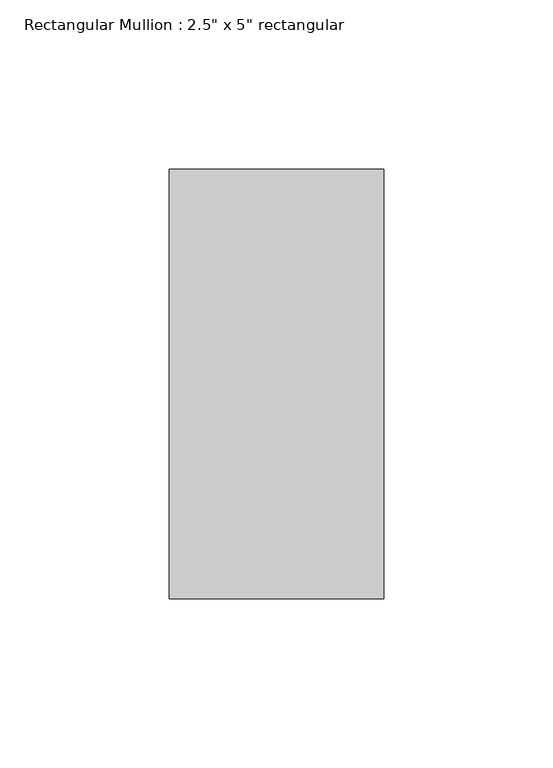
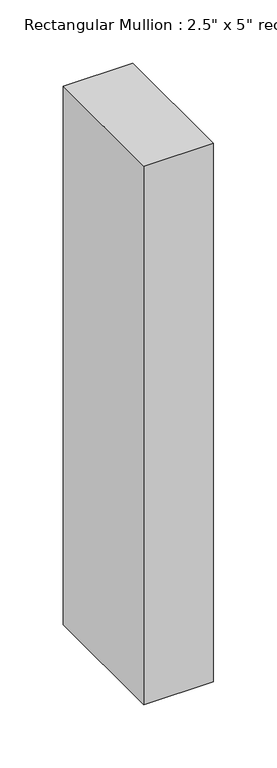
"""IFC4 building model written with IfcOpenShell, lengths in millimetres: member geometry."""

from ifc_helpers import new_model, si_unit, frame, origin, place, context, project, spatial, polyline, outline, extrude, source, transform, mapped, element, save


def member_f1b77eba(model_context):
    return source(origin(), model_context, "Body", "SweptSolid", [
        extrude(outline(polyline([(0.0, 63.5), (0.0, -63.5), (-63.5, -63.5), (-63.5, 63.5), (0.0, 63.5)])), frame((0.0, 0.0, -518.9090709), z_axis=(0.0, 0.0, 1.0), x_axis=(1.0, 0.0, 0.0)), (0.0, 0.0, 1.0), 518.9090709),
    ])


if __name__ == "__main__":
    model = new_model("IFC4")
    model_context = context("Model", 3, world=origin())
    ifc_project = project(units=[si_unit("LENGTHUNIT", "METRE", prefix="MILLI")], contexts=[model_context])
    site = spatial("IfcSite", under=ifc_project)
    building = spatial("IfcBuilding", under=site)
    placement = place(None, origin())
    member_shape = member_f1b77eba(model_context)
    element("IfcMember", 1, ObjectType="Rectangular Mullion : 2.5\" x 5\" rectangular", at=placement, inside=building, context=model_context, shape_type="MappedRepresentation", body=[
        mapped(member_shape, transform((0.0, 0.0, 0.0), x_axis=(1.0, 0.0, 0.0), y_axis=(0.0, 1.0, 0.0), z_axis=(0.0, 0.0, 1.0))),
    ])
    save(model, "model.ifc")

# Revit data of these elements
# Type "Rectangular Mullion : 2.5\" x 5\" rectangular"
#   built-in parameter 1007304 = 0.416667 (stored number, unit not read)
#   built-in parameter 1007301 = 0.104167 (stored number, unit not read)
#   built-in parameter 1007300 = 0.104167 (stored number, unit not read)
# Element 1 (IfcMember, "Rectangular Mullion : 2.5\" x 5\" rectangular")
#   Materials on its faces: "Aluminum"
# Materials
#   "Aluminum": class "Metal", colour RGB 247 247 247, transparency 0, Description = "Aluminum 6061", Cost = 0
